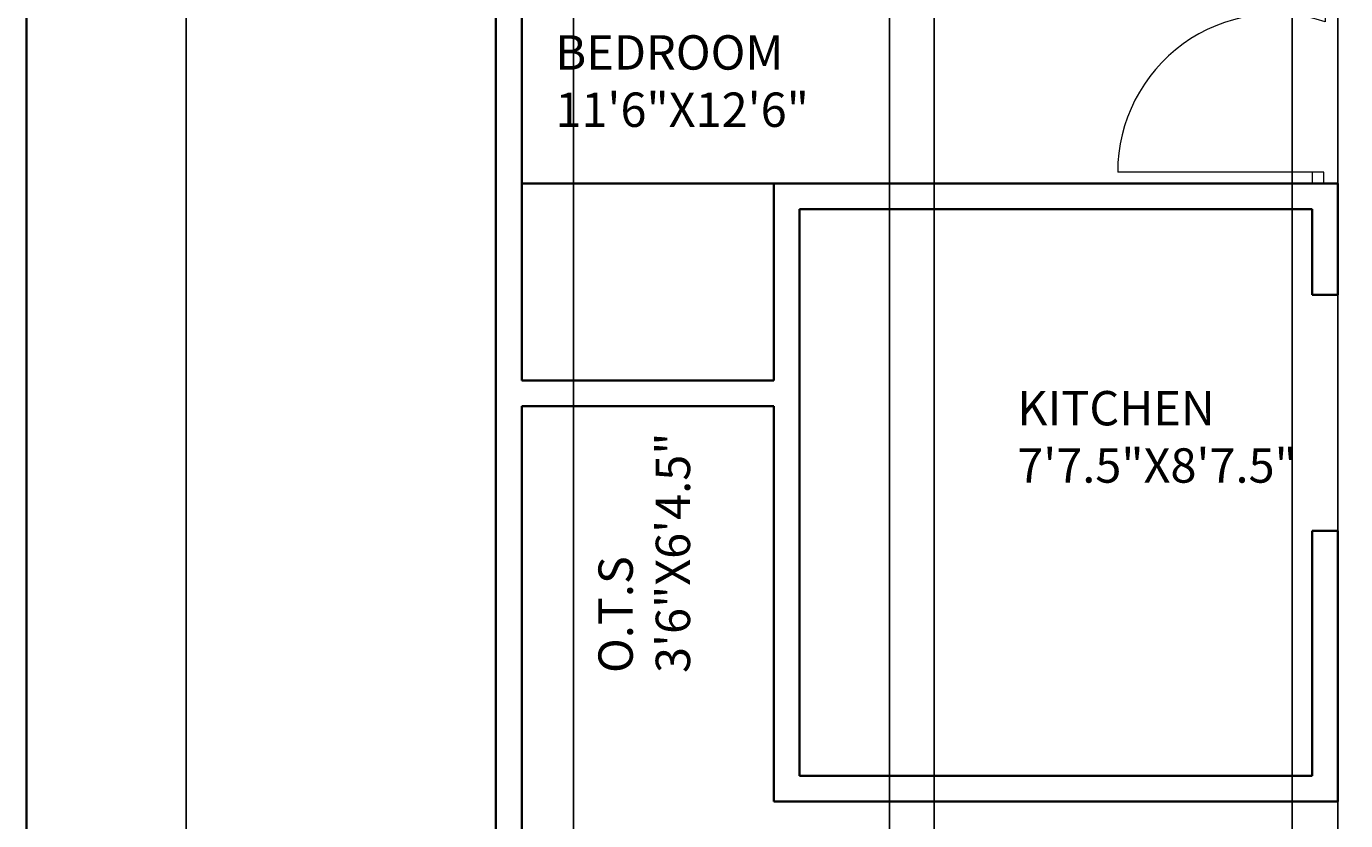
# Model space of a CAD drawing. Units: inches. Extents: x 1088 to 1703, y 668 to 1875.
# Tile 13 of 45: x 1088 to 1319, y 1572 to 1711. Entities that reach past the tile are written whole.
import ezdxf

# ---------------------------------------------------------------- set-up
doc = ezdxf.new("R2010")
doc.units = ezdxf.units.IN
for name, color, linetype, lineweight in [('A-ANNO-DIMS', 2, 'Continuous', 18), ('A-ANNO-TTLB', 7, 'Continuous', 35), ('A-AREA-IDEN', 7, 'Continuous', 18), ('A-DOOR', 4, 'Continuous', 18), ('A-WALL', 7, 'Continuous', 35)]:
    doc.layers.add(name, color=color, linetype=linetype, lineweight=lineweight)
doc.styles.get("Standard").update_dxf_attribs({"font": 'arial.ttf'})
doc.dimstyles.get("Standard").update_dxf_attribs({"dimtxt": 0.18, "dimasz": 0.18, "dimexe": 0.18, "dimexo": 0.0625, "dimgap": 0.09, "dimtad": 0, "dimtih": 1, "dimtoh": 1, "dimdec": 4, "dimzin": 0, "dimdsep": 46, "dimtxsty": 'Standard', "dimcen": 0.09, "dimadec": 0, "dimazin": 0, "dimtfac": 1, "dimtdec": 4, "dimtofl": 0, "dimtmove": 0, "dimatfit": 3, "dimfxl": 1, "dimtolj": 1, "dimtzin": 0, "dimarcsym": 0})

# ---------------------------------------------------------------- blocks, each defined once
blk = doc.blocks.new('DOOR-SWING-36')
for p, q in [((36.2, 30.23), (36.2, 28.23)), ((36, 2), (0, 2)), ((36, 0), (36, 2))]:
    blk.add_line(p, q)
blk.add_arc((27.61, 2), 27.61, 71.8583, 180)
blk = doc.blocks.new('*D29')
at = {"layer": 'A-ANNO-DIMS', "color": 0, "lineweight": -2, "transparency": 16777216}
for p, q in [((1170.28, 1803.56), (1116.11, 1803.56)), ((1116.29, 1803.38), (1116.29, 1291.85)), ((1116.29, 779.96), (1116.29, 1291.49)), ((1170.28, 779.78), (1116.11, 779.78))]:
    blk.add_line(p, q, dxfattribs=at)
at = {"layer": 'A-ANNO-DIMS', "color": 0, "transparency": 16777216}
for points in [[(1116.26, 1803.38), (1116.32, 1803.38), (1116.29, 1803.56)], [(1116.26, 779.96), (1116.32, 779.96), (1116.29, 779.78)]]:
    blk.add_solid(points, dxfattribs=at)
at = {"layer": 'Defpoints', "color": 0, "transparency": 16777216}
for p in [(1116.29, 1803.56), (1170.34, 1803.56), (1170.34, 779.78)]:
    blk.add_point(p, dxfattribs=at)
at = {"layer": 'A-ANNO-DIMS', "color": 0, "transparency": 16777216, "insert": (1116.29, 1291.67), "char_height": 0.18, "attachment_point": 5}
blk.add_mtext('\\A1;1023.8', dxfattribs=at)
blk = doc.blocks.new('*D35')
at = {"layer": 'A-ANNO-DIMS', "color": 0, "lineweight": -2, "transparency": 16777216}
for p, q in [((1183.89, 1448.1), (1183.89, 1857.79)), ((1184.07, 1857.61), (1211.07, 1857.61)), ((1238.86, 1857.61), (1211.86, 1857.61)), ((1239.04, 1448.1), (1239.04, 1857.79))]:
    blk.add_line(p, q, dxfattribs=at)
at = {"layer": 'A-ANNO-DIMS', "color": 0, "transparency": 16777216}
for points in [[(1184.07, 1857.64), (1184.07, 1857.58), (1183.89, 1857.61)], [(1238.86, 1857.64), (1238.86, 1857.58), (1239.04, 1857.61)]]:
    blk.add_solid(points, dxfattribs=at)
at = {"layer": 'Defpoints', "color": 0, "transparency": 16777216}
for p in [(1239.04, 1857.61), (1183.89, 1448.04), (1239.04, 1448.04)]:
    blk.add_point(p, dxfattribs=at)
at = {"layer": 'A-ANNO-DIMS', "color": 0, "transparency": 16777216, "insert": (1211.47, 1857.61), "char_height": 0.18, "attachment_point": 5}
blk.add_mtext('\\A1;55.15', dxfattribs=at)
blk = doc.blocks.new('*D36')
at = {"layer": 'A-ANNO-DIMS', "color": 0, "lineweight": -2, "transparency": 16777216}
for p, q in [((1246.85, 1448.35), (1246.85, 1857.79)), ((1247.03, 1857.61), (1277.78, 1857.61)), ((1309.17, 1857.61), (1278.43, 1857.61)), ((1309.35, 1448.35), (1309.35, 1857.79))]:
    blk.add_line(p, q, dxfattribs=at)
at = {"layer": 'A-ANNO-DIMS', "color": 0, "transparency": 16777216}
for points in [[(1247.03, 1857.64), (1247.03, 1857.58), (1246.85, 1857.61)], [(1309.17, 1857.64), (1309.17, 1857.58), (1309.35, 1857.61)]]:
    blk.add_solid(points, dxfattribs=at)
at = {"layer": 'Defpoints', "color": 0, "transparency": 16777216}
for p in [(1309.35, 1857.61), (1246.85, 1448.29), (1309.35, 1448.29)]:
    blk.add_point(p, dxfattribs=at)
at = {"layer": 'A-ANNO-DIMS', "color": 0, "transparency": 16777216, "insert": (1278.1, 1857.61), "char_height": 0.18, "attachment_point": 5}
blk.add_mtext('\\A1;62.5', dxfattribs=at)
blk = doc.blocks.new('*D38')
at = {"layer": 'A-ANNO-DIMS', "color": 0, "lineweight": -2, "transparency": 16777216}
for p, q in [((1317.34, 1736.94), (1317.34, 725.55)), ((1437.34, 1736.94), (1437.34, 725.55)), ((1317.52, 725.73), (1377.06, 725.73)), ((1437.16, 725.73), (1377.62, 725.73))]:
    blk.add_line(p, q, dxfattribs=at)
at = {"layer": 'A-ANNO-DIMS', "color": 0, "transparency": 16777216}
for points in [[(1317.52, 725.76), (1317.52, 725.7), (1317.34, 725.73)], [(1437.16, 725.76), (1437.16, 725.7), (1437.34, 725.73)]]:
    blk.add_solid(points, dxfattribs=at)
at = {"layer": 'Defpoints', "color": 0, "transparency": 16777216}
for p in [(1317.34, 1737.01), (1437.34, 1737.01), (1437.34, 725.73)]:
    blk.add_point(p, dxfattribs=at)
at = {"layer": 'A-ANNO-DIMS', "color": 0, "transparency": 16777216, "insert": (1377.34, 725.73), "char_height": 0.18, "attachment_point": 5}
blk.add_mtext('\\A1;120', dxfattribs=at)

msp = doc.modelspace()

# ---------------------------------------------------------------- linework, layer by layer
at = {"layer": 'A-ANNO-TTLB'}
msp.add_lwpolyline([(1088.369, 1874.677), (1703.181, 1874.677), (1703.181, 667.947), (1088.369, 667.947)], close=True, dxfattribs=at)
at = {"layer": 'A-DOOR'}
msp.add_line((1312.845, 1685.468), (1312.845, 1683.468), dxfattribs=at)
at = {"layer": 'A-WALL'}
for p, q in [((1170.345, 1803.558), (1170.345, 836.058)), ((1174.845, 1799.058), (1174.845, 1649.058)), ((1218.852, 1683.468), (1174.845, 1683.468)), ((1317.345, 1683.468), (1218.852, 1683.468)), ((1218.852, 1683.468), (1218.852, 1679.058)), ((1317.345, 1678.968), (1317.345, 1683.468)), ((1317.345, 1683.468), (1317.345, 1664.013)), ((1174.845, 1649.058), (1174.845, 1679.058)), ((1218.852, 1679.058), (1218.852, 1649.058)), ((1218.852, 1649.058), (1218.852, 1679.058)), ((1218.852, 1679.058), (1218.852, 1649.058)), ((1223.352, 1580.058), (1223.352, 1678.968)), ((1223.352, 1678.968), (1312.845, 1678.968)), ((1312.845, 1678.968), (1312.845, 1664.013)), ((1312.845, 1664.013), (1317.345, 1664.013)), ((1174.845, 1649.058), (1218.852, 1649.058)), ((1174.845, 1644.558), (1218.852, 1644.558)), ((1174.845, 1644.558), (1174.845, 1419.144)), ((1218.852, 1644.558), (1218.852, 1575.558)), ((1312.845, 1622.827), (1312.845, 1580.058)), ((1312.845, 1622.827), (1317.345, 1622.827)), ((1317.345, 1622.827), (1317.345, 1575.558)), ((1312.845, 1580.058), (1223.352, 1580.058)), ((1317.345, 1575.558), (1317.345, 1580.058)), ((1218.852, 1575.558), (1310.352, 1575.558)), ((1310.352, 1575.558), (1312.845, 1575.558)), ((1312.845, 1575.558), (1317.345, 1575.558))]:
    msp.add_line(p, q, dxfattribs=at)

# ---------------------------------------------------------------- block references
at = {"layer": 'A-DOOR'}
msp.add_blockref('DOOR-SWING-36', (1278.893, 1683.468), dxfattribs=at)

# ---------------------------------------------------------------- texts
at = {"layer": 'A-AREA-IDEN', "char_height": 6, "attachment_point": 1}
for s, width, insert in [('BEDROOM\\P11\'6"X12\'6"', 224.92883, (1180.724, 1709.345)), ('KITCHEN\\P7\'7.5"X8\'7.5"', 119.08069, (1261.351, 1647.226))]:
    msp.add_mtext_dynamic_manual_height_columns(s, width=width, gutter_width=12.5, heights=[0], dxfattribs=dict(at, insert=insert))
at = {"layer": 'A-AREA-IDEN', "insert": (1188.236, 1597.991), "char_height": 6, "attachment_point": 1, "rotation": 90}
msp.add_mtext_dynamic_manual_height_columns('O.T.S \\P3\'6"X6\'4.5"', width=122.12869, gutter_width=12.5, heights=[0], dxfattribs=at)

# ---------------------------------------------------------------- dimensions: what is measured, and where the dimension line sits
at = {"layer": 'A-ANNO-DIMS'}
for base, p1, p2, override, picture, middle in [((1239.039, 1857.608), (1183.893, 1448.04), (1239.039, 1448.04), {"dimdec": 2, "dimlfac": 1, "dimrnd": 0, "dimzin": 0, "dimdsep": 46, "dimlunit": 2}, '*D35', (1211.466, 1857.608)), ((1309.352, 1857.608), (1246.852, 1448.287), (1309.352, 1448.287), {"dimdec": 1, "dimlfac": 1, "dimrnd": 0, "dimzin": 0, "dimdsep": 46, "dimlunit": 2}, '*D36', (1278.102, 1857.608)), ((1437.345, 725.729), (1317.345, 1737.007), (1437.345, 1737.007), {"dimdec": 0, "dimlfac": 1, "dimrnd": 0, "dimzin": 0, "dimdsep": 46, "dimlunit": 2}, '*D38', (1377.345, 725.729))]:
    dim = msp.add_linear_dim(base=base, p1=p1, p2=p2, dimstyle='Standard', override=override, dxfattribs=at)
    dim.commit()
    dim.dimension.update_dxf_attribs({"geometry": picture, "text_midpoint": middle})
dim = msp.add_linear_dim(base=(1116.295, 1803.558), p1=(1170.345, 779.779), p2=(1170.345, 1803.558), angle=90, dimstyle='Standard', override={"dimdec": 1, "dimlfac": 1, "dimrnd": 0, "dimzin": 0, "dimdsep": 46, "dimlunit": 2}, dxfattribs=at)
dim.commit()
dim.dimension.update_dxf_attribs({"geometry": '*D29', "text_midpoint": (1116.295, 1291.669)})

doc.saveas('drawing.dxf')
